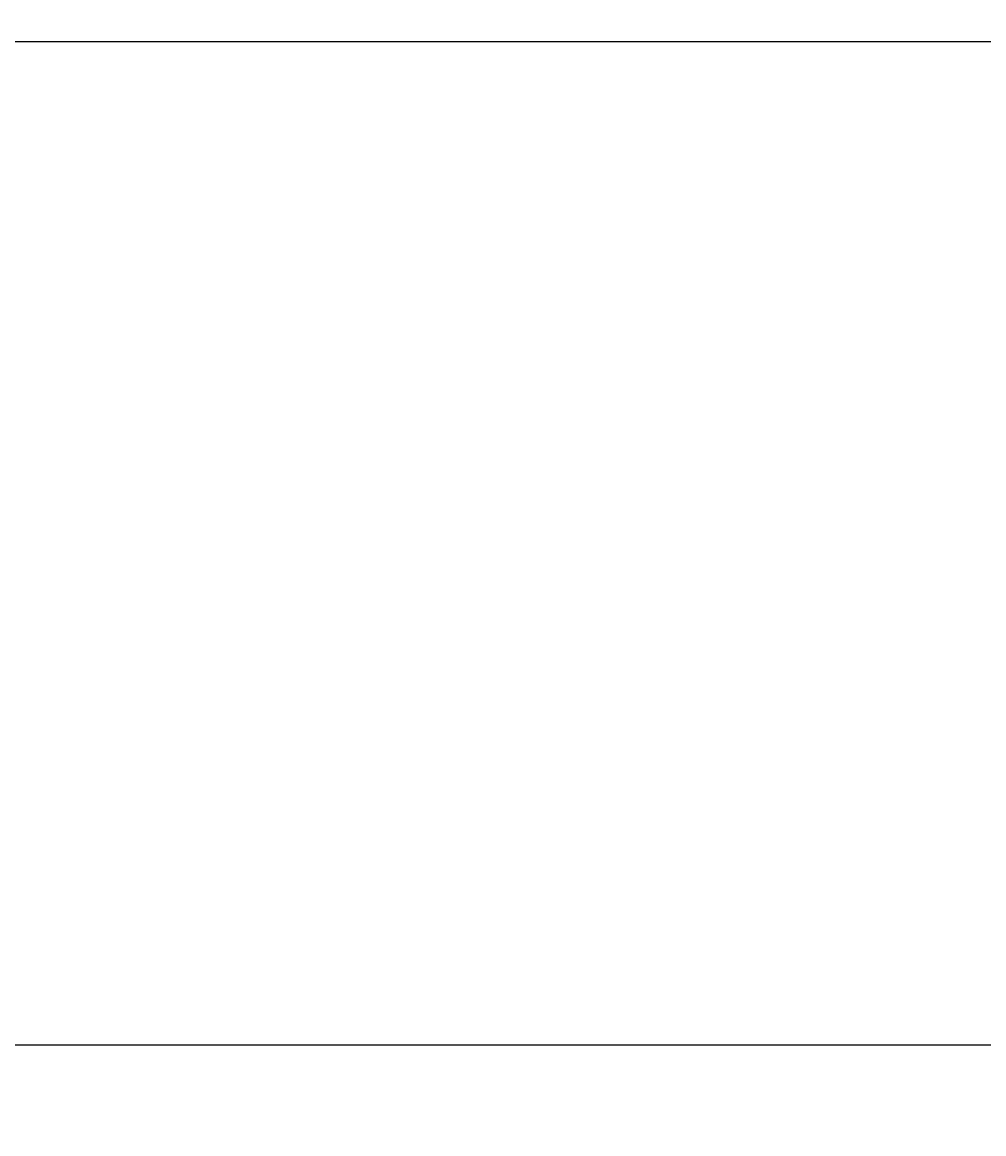
# Model space of a CAD drawing. Units: inches. Extents: x 35362 to 73946, y 43607 to 67532.
# Tile 51 of 134: x 49302 to 49711, y 46091 to 46564. Entities that reach past the tile are written whole.
import ezdxf

# ---------------------------------------------------------------- set-up
doc = ezdxf.new("R2010")
doc.units = ezdxf.units.IN
doc.header["$MEASUREMENT"] = 0
doc.layers.add('A-ANNO-DIMS', color=2, linetype='Continuous', lineweight=18)
doc.styles.get("Standard").update_dxf_attribs({"font": 'arial.ttf'})
doc.dimstyles.get("Standard").update_dxf_attribs({"dimtxt": 0.18, "dimasz": 0.18, "dimexe": 0.18, "dimexo": 0.0625, "dimgap": 0.09, "dimtad": 0, "dimtih": 1, "dimtoh": 1, "dimdec": 4, "dimzin": 0, "dimdsep": 46, "dimtxsty": 'Standard', "dimcen": 0.09, "dimadec": 0, "dimazin": 0, "dimtfac": 1, "dimtdec": 4, "dimtofl": 0, "dimtmove": 0, "dimatfit": 3, "dimfxl": 1, "dimtolj": 1, "dimtzin": 0, "dimarcsym": 0})

# ---------------------------------------------------------------- blocks, each defined once
blk = doc.blocks.new('*D5')
at = {"layer": 'A-ANNO-DIMS', "color": 0, "lineweight": -2, "transparency": 16777216}
for p, q in [((37121.95, 46919.32), (37121.95, 43606.68)), ((69871.5, 45449.83), (69871.5, 43606.68)), ((37122.13, 43606.86), (53496.29, 43606.86)), ((69871.32, 43606.86), (53497.15, 43606.86))]:
    blk.add_line(p, q, dxfattribs=at)
at = {"layer": 'A-ANNO-DIMS', "color": 0, "transparency": 16777216}
for points in [[(37122.13, 43606.89), (37122.13, 43606.83), (37121.95, 43606.86)], [(69871.32, 43606.89), (69871.32, 43606.83), (69871.5, 43606.86)]]:
    blk.add_solid(points, dxfattribs=at)
at = {"layer": 'Defpoints', "color": 0, "transparency": 16777216}
for p in [(37121.95, 46919.38), (69871.5, 45449.89), (69871.5, 43606.86)]:
    blk.add_point(p, dxfattribs=at)
at = {"layer": 'A-ANNO-DIMS', "color": 0, "transparency": 16777216, "insert": (53496.72, 43606.86), "char_height": 0.18, "attachment_point": 5}
blk.add_mtext('\\A1;32750', dxfattribs=at)
blk = doc.blocks.new('*D11')
at = {"layer": 'A-ANNO-DIMS', "color": 0, "lineweight": -2, "transparency": 16777216}
for p, q in [((47978.66, 56028.77), (47978.66, 43606.68)), ((53109.76, 56028.77), (53109.76, 43606.68)), ((47978.84, 43606.86), (50543.87, 43606.86)), ((53109.58, 43606.86), (50544.55, 43606.86))]:
    blk.add_line(p, q, dxfattribs=at)
at = {"layer": 'A-ANNO-DIMS', "color": 0, "transparency": 16777216}
for points in [[(47978.84, 43606.89), (47978.84, 43606.83), (47978.66, 43606.86)], [(53109.58, 43606.89), (53109.58, 43606.83), (53109.76, 43606.86)]]:
    blk.add_solid(points, dxfattribs=at)
at = {"layer": 'Defpoints', "color": 0, "transparency": 16777216}
for p in [(47978.66, 56028.84), (53109.76, 56028.84), (53109.76, 43606.86)]:
    blk.add_point(p, dxfattribs=at)
at = {"layer": 'A-ANNO-DIMS', "color": 0, "transparency": 16777216, "insert": (50544.21, 43606.86), "char_height": 0.18, "attachment_point": 5}
blk.add_mtext('\\A1;5131', dxfattribs=at)
blk = doc.blocks.new('*D13')
at = {"layer": 'A-ANNO-DIMS', "color": 0, "lineweight": -2, "transparency": 16777216}
for p, q in [((48373.49, 51694.02), (48373.49, 43606.68)), ((51029.04, 51694.02), (51029.04, 43606.68)), ((48373.67, 43606.86), (49700.8, 43606.86)), ((51028.86, 43606.86), (49701.73, 43606.86))]:
    blk.add_line(p, q, dxfattribs=at)
at = {"layer": 'A-ANNO-DIMS', "color": 0, "transparency": 16777216}
for points in [[(48373.67, 43606.89), (48373.67, 43606.83), (48373.49, 43606.86)], [(51028.86, 43606.89), (51028.86, 43606.83), (51029.04, 43606.86)]]:
    blk.add_solid(points, dxfattribs=at)
at = {"layer": 'Defpoints', "color": 0, "transparency": 16777216}
for p in [(48373.49, 51694.09), (51029.04, 51694.09), (51029.04, 43606.86)]:
    blk.add_point(p, dxfattribs=at)
at = {"layer": 'A-ANNO-DIMS', "color": 0, "transparency": 16777216, "insert": (49701.27, 43606.86), "char_height": 0.18, "attachment_point": 5}
blk.add_mtext('\\A1;2655.6', dxfattribs=at)
blk = doc.blocks.new('*D67')
at = {"layer": 'A-ANNO-DIMS', "color": 0, "lineweight": -2, "transparency": 16777216}
for p, q in [((56873.54, 53351.53), (35361.77, 53351.53)), ((35361.95, 53351.35), (35361.95, 49400.89)), ((35361.95, 45450.07), (35361.95, 49400.53)), ((53793.58, 45449.89), (35361.77, 45449.89))]:
    blk.add_line(p, q, dxfattribs=at)
at = {"layer": 'A-ANNO-DIMS', "color": 0, "transparency": 16777216}
for points in [[(35361.92, 53351.35), (35361.98, 53351.35), (35361.95, 53351.53)], [(35361.92, 45450.07), (35361.98, 45450.07), (35361.95, 45449.89)]]:
    blk.add_solid(points, dxfattribs=at)
at = {"layer": 'Defpoints', "color": 0, "transparency": 16777216}
for p in [(35361.95, 53351.53), (56873.6, 53351.53), (53793.64, 45449.89)]:
    blk.add_point(p, dxfattribs=at)
at = {"layer": 'A-ANNO-DIMS', "color": 0, "transparency": 16777216, "insert": (35361.95, 49400.71), "char_height": 0.18, "attachment_point": 5}
blk.add_mtext('\\A1;7901.6', dxfattribs=at)
blk = doc.blocks.new('*D76')
at = {"layer": 'A-ANNO-DIMS', "color": 0, "lineweight": -2, "transparency": 16777216}
for p, q in [((54052.84, 46555.29), (35361.77, 46555.29)), ((35361.95, 46555.11), (35361.95, 46342.27)), ((35361.95, 46129.06), (35361.95, 46341.9)), ((53793.58, 46128.88), (35361.77, 46128.88))]:
    blk.add_line(p, q, dxfattribs=at)
at = {"layer": 'A-ANNO-DIMS', "color": 0, "transparency": 16777216}
for points in [[(35361.92, 46555.11), (35361.98, 46555.11), (35361.95, 46555.29)], [(35361.92, 46129.06), (35361.98, 46129.06), (35361.95, 46128.88)]]:
    blk.add_solid(points, dxfattribs=at)
at = {"layer": 'Defpoints', "color": 0, "transparency": 16777216}
for p in [(35361.95, 46555.29), (54052.9, 46555.29), (53793.64, 46128.88)]:
    blk.add_point(p, dxfattribs=at)
at = {"layer": 'A-ANNO-DIMS', "color": 0, "transparency": 16777216, "insert": (35361.95, 46342.09), "char_height": 0.18, "attachment_point": 5}
blk.add_mtext('\\A1;426.4', dxfattribs=at)
blk = doc.blocks.new('*D90')
at = {"layer": 'A-ANNO-DIMS', "color": 0, "lineweight": -2, "transparency": 16777216}
for p, q in [((53707.72, 47291.29), (35361.77, 47291.29)), ((35361.95, 47291.11), (35361.95, 46710.26)), ((35361.95, 46129.06), (35361.95, 46709.9)), ((53793.58, 46128.88), (35361.77, 46128.88))]:
    blk.add_line(p, q, dxfattribs=at)
at = {"layer": 'A-ANNO-DIMS', "color": 0, "transparency": 16777216}
for points in [[(35361.92, 47291.11), (35361.98, 47291.11), (35361.95, 47291.29)], [(35361.92, 46129.06), (35361.98, 46129.06), (35361.95, 46128.88)]]:
    blk.add_solid(points, dxfattribs=at)
at = {"layer": 'Defpoints', "color": 0, "transparency": 16777216}
for p in [(53707.78, 47291.29), (35361.95, 46128.88), (53793.64, 46128.88)]:
    blk.add_point(p, dxfattribs=at)
at = {"layer": 'A-ANNO-DIMS', "color": 0, "transparency": 16777216, "insert": (35361.95, 46710.08), "char_height": 0.18, "attachment_point": 5}
blk.add_mtext('\\A1;1162.4', dxfattribs=at)

msp = doc.modelspace()

# ---------------------------------------------------------------- dimensions: what is measured, and where the dimension line sits
at = {"layer": 'A-ANNO-DIMS'}
for base, p1, p2, override, picture, middle in [((53109.76, 43606.859), (47978.665, 56028.836), (53109.76, 56028.836), {"dimdec": 0, "dimlfac": 1, "dimrnd": 0, "dimzin": 0, "dimdsep": 46, "dimlunit": 2}, '*D11', (50544.212, 43606.859)), ((51029.043, 43606.859), (48373.492, 51694.087), (51029.043, 51694.087), {"dimdec": 1, "dimlfac": 1, "dimrnd": 0, "dimzin": 0, "dimdsep": 46, "dimlunit": 2}, '*D13', (49701.267, 43606.859)), ((69871.496, 43606.859), (37121.949, 46919.381), (69871.496, 45449.894), {"dimdec": 0, "dimlfac": 1, "dimrnd": 0, "dimzin": 0, "dimdsep": 46, "dimlunit": 2}, '*D5', (53496.723, 43606.859))]:
    dim = msp.add_linear_dim(base=base, p1=p1, p2=p2, dimstyle='Standard', override=override, dxfattribs=at)
    dim.commit()
    dim.dimension.update_dxf_attribs({"geometry": picture, "text_midpoint": middle})
for base, p1, p2, picture, middle in [((35361.949, 53351.529), (53793.638, 45449.894), (56873.602, 53351.529), '*D67', (35361.949, 49400.712)), ((35361.949, 46128.878), (53707.781, 47291.285), (53793.638, 46128.878), '*D90', (35361.949, 46710.081)), ((35361.949, 46555.293), (53793.638, 46128.878), (54052.899, 46555.293), '*D76', (35361.949, 46342.086))]:
    dim = msp.add_linear_dim(base=base, p1=p1, p2=p2, angle=90, dimstyle='Standard', override={"dimdec": 1, "dimlfac": 1, "dimrnd": 0, "dimzin": 0, "dimdsep": 46, "dimlunit": 2}, dxfattribs=at)
    dim.commit()
    dim.dimension.update_dxf_attribs({"geometry": picture, "text_midpoint": middle})

doc.saveas('drawing.dxf')
